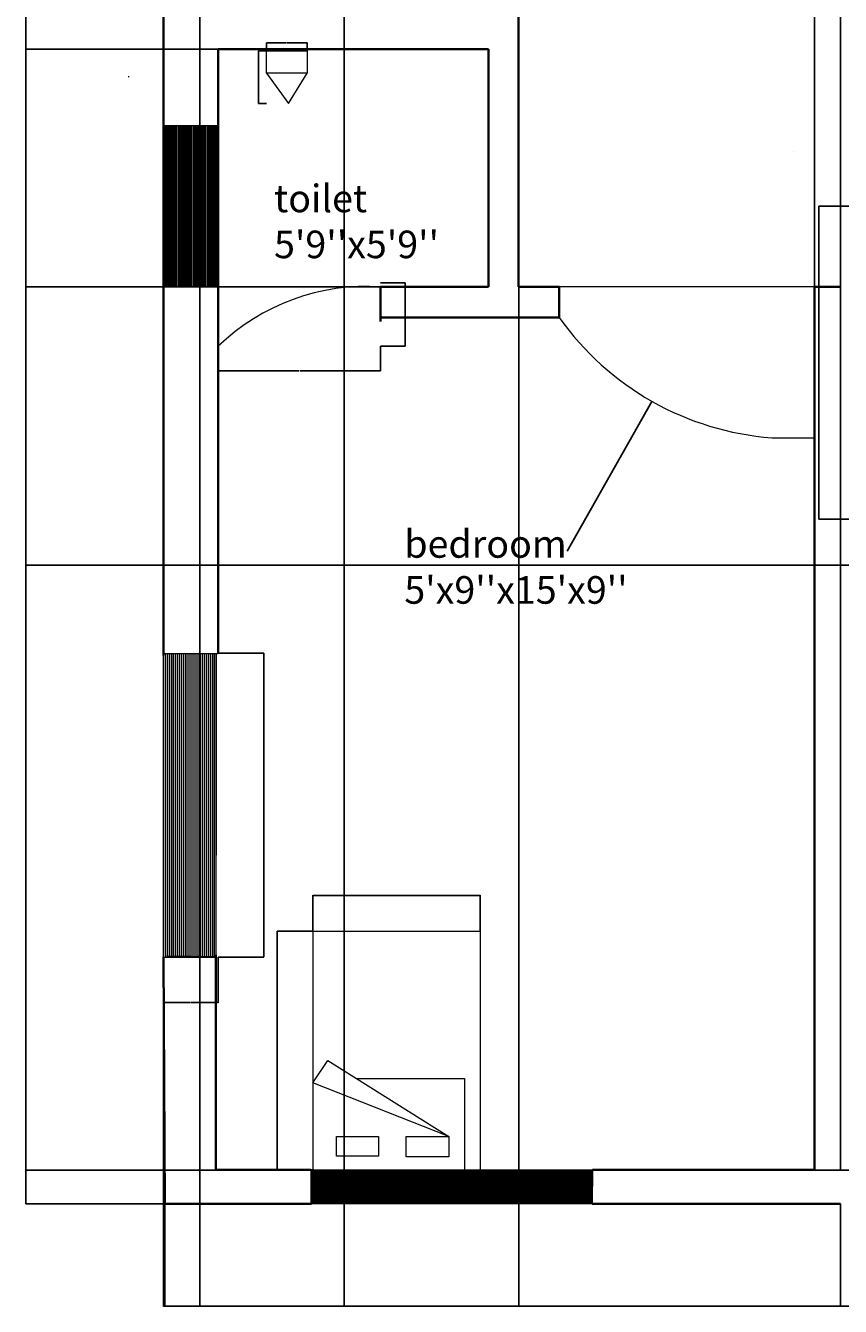
# Model space of a CAD drawing. Units: millimetres. Extents: x 1942 to 12281, y -2698 to 3078.
# Tile 1 of 6: x 1942 to 4011, y -2698 to 552. Entities that reach past the tile are written whole.
import ezdxf

# ---------------------------------------------------------------- set-up
doc = ezdxf.new("R2010")
doc.units = ezdxf.units.MM
for name, color, linetype, lineweight in [('A-ANNO-DIMS', 2, 'Continuous', 18), ('A-AREA-IDEN', 3, 'Continuous', 18), ('A-DETL-REF', 8, 'Continuous', 13), ('A-DOOR', 4, 'Continuous', 18), ('A-FLOR-FIXT', 9, 'Continuous', 18), ('A-FURN', 8, 'Continuous', 18), ('A-GLAZ', 4, 'Continuous', 18), ('A-GLAZ-PATT', 9, 'Continuous', 13), ('A-WALL', 7, 'Continuous', 35)]:
    doc.layers.add(name, color=color, linetype=linetype, lineweight=lineweight)
doc.styles.get("Standard").update_dxf_attribs({"font": 'arial.ttf'})
doc.dimstyles.get("Standard").update_dxf_attribs({"dimtxt": 0.18, "dimasz": 0.18, "dimexe": 0.18, "dimexo": 0.0625, "dimgap": 0.09, "dimtad": 0, "dimtih": 1, "dimtoh": 1, "dimdec": 4, "dimzin": 0, "dimdsep": 46, "dimtxsty": 'Standard', "dimcen": 0.09, "dimadec": 0, "dimazin": 0, "dimtfac": 1, "dimtdec": 4, "dimtofl": 0, "dimtmove": 0, "dimatfit": 3, "dimfxl": 1, "dimtolj": 1, "dimtzin": 0, "dimarcsym": 0})

# ---------------------------------------------------------------- blocks, each defined once
blk = doc.blocks.new('BED-PILLOWS')
for p, q in [((0, 605.9), (424.9, 605.9)), ((0, 605.9), (0, 0)), ((424.9, 605.9), (424.9, 0)), ((0, 221), (38.1, 277.4)), ((38.1, 277.4), (344.8, 84.6)), ((109.8, 232.4), (384.7, 232.4)), ((384.7, 232.4), (384.7, 0)), ((344.8, 84.6), (0, 221)), ((0, 0), (0, 0))]:
    blk.add_line(p, q)
for points in [[(59.7, 84.6), (166.4, 84.6), (166.4, 35.4), (59.7, 35.4)], [(236.8, 84.6), (344.8, 84.6), (344.8, 33.1), (236.8, 33.1)]]:
    blk.add_lwpolyline(points, close=True)
blk = doc.blocks.new('WC-TAPERED-LONG')
for p, q in [((0, 77), (55.9, 0)), ((55.9, 0), (103.2, 77))]:
    blk.add_line(p, q)
blk.add_lwpolyline([(0, 134), (103.2, 134), (103.2, 77), (0, 77)], close=True)
blk = doc.blocks.new('DOOR-BEDROOM')
for p, q in [((648.7, 382.9), (0, 382.9)), ((539.8, 0), (648.7, 0))]:
    blk.add_line(p, q)
blk.add_arc((594.3, 726.1), 728.1, 215.2982, 265.7132)
blk = doc.blocks.new('DOOR-WC-BEDROOM')
blk.add_arc((376.5, -390), 542.1, 86.1851, 133.9877)
blk = doc.blocks.new('WIN-BEDROOM-SIDE')
for p, q in [((138.7, 769.7), (0, 769.7)), ((0, 765.5), (0, 0.1)), ((132.6, 771), (132.6, 5.6)), ((0, 0.1), (132.6, 0.1)), ((8.8, 3.3), (132.6, 1.4)), ((95.6, 3.3), (78.2, 0))]:
    blk.add_line(p, q)
blk = doc.blocks.new('WIN-BEDROOM-END')
for p, q in [((0, 85.7), (0, 0)), ((0, 85.7), (430, 85.7)), ((714.9, 85.7), (714.3, 0)), ((714.3, 0), (1.8, 0))]:
    blk.add_line(p, q)
blk = doc.blocks.new('*D26')
at = {"layer": 'A-ANNO-DIMS', "color": 0, "lineweight": -2, "transparency": 16777216}
for p, q in [((2671.4, -1745.7), (2580.4, -1745.7)), ((2580.5, -1745.8), (2580.5, -2048.4)), ((2580.5, -2351.4), (2580.5, -2048.8)), ((2671.4, -2351.5), (2580.4, -2351.5))]:
    blk.add_line(p, q, dxfattribs=at)
at = {"layer": 'A-ANNO-DIMS', "color": 0, "transparency": 16777216}
for points in [[(2580.5, -1745.8), (2580.6, -1745.8), (2580.5, -1745.7)], [(2580.5, -2351.4), (2580.6, -2351.4), (2580.5, -2351.5)]]:
    blk.add_solid(points, dxfattribs=at)
at = {"layer": 'Defpoints', "color": 0, "transparency": 16777216}
for p in [(2580.5, -1745.7), (2671.4, -1745.7), (2671.4, -2351.5)]:
    blk.add_point(p, dxfattribs=at)
at = {"layer": 'A-ANNO-DIMS', "color": 0, "transparency": 16777216, "insert": (2580.5, -2048.6), "char_height": 0.18, "attachment_point": 5}
blk.add_mtext('\\A1;BED 606 TYP.', dxfattribs=at)
blk = doc.blocks.new('*D27')
at = {"layer": 'A-ANNO-DIMS', "color": 0, "lineweight": -2, "transparency": 16777216}
for p, q in [((2671.4, -1745.6), (2671.4, -1654.6)), ((2671.6, -1654.8), (2883.3, -1654.8)), ((3096.2, -1654.8), (2884.5, -1654.8)), ((3096.3, -1745.6), (3096.3, -1654.6))]:
    blk.add_line(p, q, dxfattribs=at)
at = {"layer": 'A-ANNO-DIMS', "color": 0, "transparency": 16777216}
for points in [[(2671.6, -1654.8), (2671.6, -1654.8), (2671.4, -1654.8)], [(3096.2, -1654.8), (3096.2, -1654.8), (3096.3, -1654.8)]]:
    blk.add_solid(points, dxfattribs=at)
at = {"layer": 'Defpoints', "color": 0, "transparency": 16777216}
for p in [(3096.3, -1654.8), (2671.4, -1745.7), (3096.3, -1745.7)]:
    blk.add_point(p, dxfattribs=at)
at = {"layer": 'A-ANNO-DIMS', "color": 0, "transparency": 16777216, "insert": (2883.9, -1654.8), "char_height": 0.18, "attachment_point": 5}
blk.add_mtext('\\A1;425 TYP.', dxfattribs=at)
blk = doc.blocks.new('*D29')
at = {"layer": 'A-ANNO-DIMS', "color": 0, "lineweight": -2, "transparency": 16777216}
for p, q in [((4101.3, 94.1), (3956.1, 94.1)), ((3956.3, 94), (3956.3, -302.8)), ((3956.3, -700), (3956.3, -303.2)), ((4101.3, -700.2), (3956.1, -700.2))]:
    blk.add_line(p, q, dxfattribs=at)
at = {"layer": 'A-ANNO-DIMS', "color": 0, "transparency": 16777216}
for points in [[(3956.3, 94), (3956.3, 94), (3956.3, 94.1)], [(3956.3, -700), (3956.3, -700), (3956.3, -700.2)]]:
    blk.add_solid(points, dxfattribs=at)
at = {"layer": 'Defpoints', "color": 0, "transparency": 16777216}
for p in [(3956.3, 94.1), (4101.4, 94.1), (4101.4, -700.2)]:
    blk.add_point(p, dxfattribs=at)
at = {"layer": 'A-ANNO-DIMS', "color": 0, "transparency": 16777216, "insert": (3956.3, -303), "char_height": 0.18, "attachment_point": 5}
blk.add_mtext('\\A1;794 TYP.', dxfattribs=at)
blk = doc.blocks.new('*D36')
at = {"layer": 'A-ANNO-DIMS', "color": 0, "lineweight": -2, "transparency": 16777216}
for p, q in [((2553.4, 488.5), (2533.2, 488.5)), ((2533.3, 488.3), (2533.3, 421.7)), ((2533.3, 354.7), (2533.3, 421.3)), ((2553.4, 354.5), (2533.2, 354.5))]:
    blk.add_line(p, q, dxfattribs=at)
at = {"layer": 'A-ANNO-DIMS', "color": 0, "transparency": 16777216}
for points in [[(2533.3, 488.3), (2533.4, 488.3), (2533.3, 488.5)], [(2533.3, 354.7), (2533.4, 354.7), (2533.3, 354.5)]]:
    blk.add_solid(points, dxfattribs=at)
at = {"layer": 'Defpoints', "color": 0, "transparency": 16777216}
for p in [(2533.3, 488.5), (2553.4, 488.5), (2553.4, 354.5)]:
    blk.add_point(p, dxfattribs=at)
at = {"layer": 'A-ANNO-DIMS', "color": 0, "transparency": 16777216, "insert": (2533.3, 421.5), "char_height": 0.18, "attachment_point": 5}
blk.add_mtext('\\A1;WC 134 TYP.', dxfattribs=at)
blk = doc.blocks.new('*D37')
at = {"layer": 'A-ANNO-DIMS', "color": 0, "lineweight": -2, "transparency": 16777216}
for p, q in [((2553.4, 488.5), (2553.4, 508.7)), ((2553.6, 508.6), (2604.4, 508.6)), ((2656.4, 508.6), (2605.6, 508.6)), ((2656.6, 488.5), (2656.6, 508.7))]:
    blk.add_line(p, q, dxfattribs=at)
at = {"layer": 'A-ANNO-DIMS', "color": 0, "transparency": 16777216}
for points in [[(2553.6, 508.6), (2553.6, 508.5), (2553.4, 508.6)], [(2656.4, 508.6), (2656.4, 508.5), (2656.6, 508.6)]]:
    blk.add_solid(points, dxfattribs=at)
at = {"layer": 'Defpoints', "color": 0, "transparency": 16777216}
for p in [(2553.4, 488.5), (2656.6, 508.6), (2656.6, 488.5)]:
    blk.add_point(p, dxfattribs=at)
at = {"layer": 'A-ANNO-DIMS', "color": 0, "transparency": 16777216, "insert": (2605, 508.6), "char_height": 0.18, "attachment_point": 5}
blk.add_mtext('\\A1;103 TYP.', dxfattribs=at)
blk = doc.blocks.new('*D44')
at = {"layer": 'A-ANNO-DIMS', "color": 0, "lineweight": -2, "transparency": 16777216}
for p, q in [((2430.7, -261.5), (2430.7, -323.5)), ((2843.3, -261.5), (2843.3, -323.5)), ((2430.9, -323.3), (2635.7, -323.3)), ((2843.1, -323.3), (2638.3, -323.3))]:
    blk.add_line(p, q, dxfattribs=at)
at = {"layer": 'A-ANNO-DIMS', "color": 0, "transparency": 16777216}
for points in [[(2430.9, -323.3), (2430.9, -323.4), (2430.7, -323.3)], [(2843.1, -323.3), (2843.1, -323.4), (2843.3, -323.3)]]:
    blk.add_solid(points, dxfattribs=at)
at = {"layer": 'Defpoints', "color": 0, "transparency": 16777216}
for p in [(2430.7, -261.5), (2843.3, -261.5), (2843.3, -323.3)]:
    blk.add_point(p, dxfattribs=at)
at = {"layer": 'A-ANNO-DIMS', "color": 0, "transparency": 16777216, "insert": (2637, -323.3), "char_height": 0.18, "attachment_point": 5}
blk.add_mtext('\\A1;WC DOOR 413 TYP.', dxfattribs=at)
blk = doc.blocks.new('*D45')
at = {"layer": 'A-ANNO-DIMS', "color": 0, "lineweight": -2, "transparency": 16777216}
for p, q in [((2843.3, -100.4), (2905.3, -100.4)), ((2905.2, -100.6), (2905.2, -180.8)), ((2905.2, -261.3), (2905.2, -181.1)), ((2843.3, -261.5), (2905.3, -261.5))]:
    blk.add_line(p, q, dxfattribs=at)
at = {"layer": 'A-ANNO-DIMS', "color": 0, "transparency": 16777216}
for points in [[(2905.1, -100.6), (2905.2, -100.6), (2905.2, -100.4)], [(2905.1, -261.3), (2905.2, -261.3), (2905.2, -261.5)]]:
    blk.add_solid(points, dxfattribs=at)
at = {"layer": 'Defpoints', "color": 0, "transparency": 16777216}
for p in [(2843.3, -100.4), (2905.2, -100.4), (2843.3, -261.5)]:
    blk.add_point(p, dxfattribs=at)
at = {"layer": 'A-ANNO-DIMS', "color": 0, "transparency": 16777216, "insert": (2905.2, -180.9), "char_height": 0.18, "attachment_point": 5}
blk.add_mtext('\\A1;161 TYP.', dxfattribs=at)
blk = doc.blocks.new('*D64')
at = {"layer": 'A-ANNO-DIMS', "color": 0, "lineweight": -2, "transparency": 16777216}
for p, q in [((2430.8, -1040.2), (2546.6, -1040.2)), ((2546.4, -1040.4), (2546.4, -1425.5)), ((2546.4, -1811), (2546.4, -1425.9)), ((2430.8, -1811.2), (2546.6, -1811.2))]:
    blk.add_line(p, q, dxfattribs=at)
at = {"layer": 'A-ANNO-DIMS', "color": 0, "transparency": 16777216}
for points in [[(2546.3, -1040.4), (2546.4, -1040.4), (2546.4, -1040.2)], [(2546.3, -1811), (2546.4, -1811), (2546.4, -1811.2)]]:
    blk.add_solid(points, dxfattribs=at)
at = {"layer": 'Defpoints', "color": 0, "transparency": 16777216}
for p in [(2430.7, -1040.2), (2546.4, -1040.2), (2430.7, -1811.2)]:
    blk.add_point(p, dxfattribs=at)
at = {"layer": 'A-ANNO-DIMS', "color": 0, "transparency": 16777216, "insert": (2546.4, -1425.7), "char_height": 0.18, "attachment_point": 5}
blk.add_mtext('\\A1;W3 771 TYP.', dxfattribs=at)
blk = doc.blocks.new('*D65')
at = {"layer": 'A-ANNO-DIMS', "color": 0, "lineweight": -2, "transparency": 16777216}
for p, q in [((2292.1, -1811.3), (2292.1, -1927)), ((2430.7, -1811.3), (2430.7, -1927)), ((2292.2, -1926.8), (2360.8, -1926.8)), ((2430.5, -1926.8), (2362, -1926.8))]:
    blk.add_line(p, q, dxfattribs=at)
at = {"layer": 'A-ANNO-DIMS', "color": 0, "transparency": 16777216}
for points in [[(2292.2, -1926.8), (2292.2, -1926.9), (2292.1, -1926.8)], [(2430.5, -1926.8), (2430.5, -1926.9), (2430.7, -1926.8)]]:
    blk.add_solid(points, dxfattribs=at)
at = {"layer": 'Defpoints', "color": 0, "transparency": 16777216}
for p in [(2292.1, -1811.2), (2430.7, -1811.2), (2430.7, -1926.8)]:
    blk.add_point(p, dxfattribs=at)
at = {"layer": 'A-ANNO-DIMS', "color": 0, "transparency": 16777216, "insert": (2361.4, -1926.8), "char_height": 0.18, "attachment_point": 5}
blk.add_mtext('\\A1;139 TYP.', dxfattribs=at)
blk = doc.blocks.new('*D72')
at = {"layer": 'A-ANNO-DIMS', "color": 0, "lineweight": -2, "transparency": 16777216}
for p, q in [((2295.7, -2437.3), (2295.7, -2697.7)), ((4010.7, -2437.3), (4010.7, -2697.7)), ((2295.8, -2697.5), (3152.8, -2697.5)), ((4010.5, -2697.5), (3153.5, -2697.5))]:
    blk.add_line(p, q, dxfattribs=at)
at = {"layer": 'A-ANNO-DIMS', "color": 0, "transparency": 16777216}
for points in [[(2295.8, -2697.5), (2295.8, -2697.5), (2295.7, -2697.5)], [(4010.5, -2697.5), (4010.5, -2697.5), (4010.7, -2697.5)]]:
    blk.add_solid(points, dxfattribs=at)
at = {"layer": 'Defpoints', "color": 0, "transparency": 16777216}
for p in [(2295.7, -2437.2), (4010.7, -2437.2), (4010.7, -2697.5)]:
    blk.add_point(p, dxfattribs=at)
at = {"layer": 'A-ANNO-DIMS', "color": 0, "transparency": 16777216, "insert": (3153.2, -2697.5), "char_height": 0.18, "attachment_point": 5}
blk.add_mtext('\\A1;1715', dxfattribs=at)
blk = doc.blocks.new('*D73')
at = {"layer": 'A-ANNO-DIMS', "color": 0, "lineweight": -2, "transparency": 16777216}
for p, q in [((4010.7, -2437.3), (4010.7, -2697.7)), ((6894.1, -2437.3), (6894.1, -2697.7)), ((4010.9, -2697.5), (5451.9, -2697.5)), ((6893.9, -2697.5), (5452.9, -2697.5))]:
    blk.add_line(p, q, dxfattribs=at)
at = {"layer": 'A-ANNO-DIMS', "color": 0, "transparency": 16777216}
for points in [[(4010.9, -2697.5), (4010.9, -2697.5), (4010.7, -2697.5)], [(6893.9, -2697.5), (6893.9, -2697.5), (6894.1, -2697.5)]]:
    blk.add_solid(points, dxfattribs=at)
at = {"layer": 'Defpoints', "color": 0, "transparency": 16777216}
for p in [(4010.7, -2437.2), (6894.1, -2437.2), (6894.1, -2697.5)]:
    blk.add_point(p, dxfattribs=at)
at = {"layer": 'A-ANNO-DIMS', "color": 0, "transparency": 16777216, "insert": (5452.4, -2697.5), "char_height": 0.18, "attachment_point": 5}
blk.add_mtext('\\A1;2883.4', dxfattribs=at)
blk = doc.blocks.new('*D77')
at = {"layer": 'A-ANNO-DIMS', "color": 0, "lineweight": -2, "transparency": 16777216}
for p, q in [((2292, 1112.1), (1942, 1112.1)), ((1942.2, 1111.9), (1942.2, 802.3)), ((1942.2, 492.4), (1942.2, 801.9)), ((3116.8, 492.2), (1942, 492.2))]:
    blk.add_line(p, q, dxfattribs=at)
at = {"layer": 'A-ANNO-DIMS', "color": 0, "transparency": 16777216}
for points in [[(1942.2, 1111.9), (1942.2, 1111.9), (1942.2, 1112.1)], [(1942.2, 492.4), (1942.2, 492.4), (1942.2, 492.2)]]:
    blk.add_solid(points, dxfattribs=at)
at = {"layer": 'Defpoints', "color": 0, "transparency": 16777216}
for p in [(1942.2, 1112.1), (2292.1, 1112.1), (3116.8, 492.2)]:
    blk.add_point(p, dxfattribs=at)
at = {"layer": 'A-ANNO-DIMS', "color": 0, "transparency": 16777216, "insert": (1942.2, 802.1), "char_height": 0.18, "attachment_point": 5}
blk.add_mtext('\\A1;619.9', dxfattribs=at)
blk = doc.blocks.new('*D78')
at = {"layer": 'A-ANNO-DIMS', "color": 0, "lineweight": -2, "transparency": 16777216}
for p, q in [((3116.8, 492.2), (1942, 492.2)), ((1942.2, 492), (1942.2, 191)), ((1942.2, -110.4), (1942.2, 190.6)), ((3116.8, -110.6), (1942, -110.6))]:
    blk.add_line(p, q, dxfattribs=at)
at = {"layer": 'A-ANNO-DIMS', "color": 0, "transparency": 16777216}
for points in [[(1942.2, 492), (1942.2, 492), (1942.2, 492.2)], [(1942.2, -110.4), (1942.2, -110.4), (1942.2, -110.6)]]:
    blk.add_solid(points, dxfattribs=at)
at = {"layer": 'Defpoints', "color": 0, "transparency": 16777216}
for p in [(1942.2, 492.2), (3116.8, 492.2), (3116.8, -110.6)]:
    blk.add_point(p, dxfattribs=at)
at = {"layer": 'A-ANNO-DIMS', "color": 0, "transparency": 16777216, "insert": (1942.2, 190.8), "char_height": 0.18, "attachment_point": 5}
blk.add_mtext('\\A1;602.8', dxfattribs=at)
blk = doc.blocks.new('*D79')
at = {"layer": 'A-ANNO-DIMS', "color": 0, "lineweight": -2, "transparency": 16777216}
for p, q in [((3116.8, -110.6), (1942, -110.6)), ((1942.2, -110.8), (1942.2, -1273.7)), ((1942.2, -2437.1), (1942.2, -1274.1)), ((2295.6, -2437.2), (1942, -2437.2))]:
    blk.add_line(p, q, dxfattribs=at)
at = {"layer": 'A-ANNO-DIMS', "color": 0, "transparency": 16777216}
for points in [[(1942.2, -110.8), (1942.2, -110.8), (1942.2, -110.6)], [(1942.2, -2437.1), (1942.2, -2437.1), (1942.2, -2437.2)]]:
    blk.add_solid(points, dxfattribs=at)
at = {"layer": 'Defpoints', "color": 0, "transparency": 16777216}
for p in [(1942.2, -110.6), (3116.8, -110.6), (2295.7, -2437.2)]:
    blk.add_point(p, dxfattribs=at)
at = {"layer": 'A-ANNO-DIMS', "color": 0, "transparency": 16777216, "insert": (1942.2, -1273.9), "char_height": 0.18, "attachment_point": 5}
blk.add_mtext('\\A1;2326.6', dxfattribs=at)
blk = doc.blocks.new('*D80')
at = {"layer": 'A-ANNO-DIMS', "color": 0, "lineweight": -2, "transparency": 16777216}
for p, q in [((2292.1, 1112), (2292.1, -2697.7)), ((3193.8, 769.3), (3193.8, -2697.7)), ((2292.2, -2697.5), (2742.5, -2697.5)), ((3193.6, -2697.5), (2743.3, -2697.5))]:
    blk.add_line(p, q, dxfattribs=at)
at = {"layer": 'A-ANNO-DIMS', "color": 0, "transparency": 16777216}
for points in [[(2292.2, -2697.5), (2292.2, -2697.5), (2292.1, -2697.5)], [(3193.6, -2697.5), (3193.6, -2697.5), (3193.8, -2697.5)]]:
    blk.add_solid(points, dxfattribs=at)
at = {"layer": 'Defpoints', "color": 0, "transparency": 16777216}
for p in [(2292.1, 1112.1), (3193.8, 769.4), (3193.8, -2697.5)]:
    blk.add_point(p, dxfattribs=at)
at = {"layer": 'A-ANNO-DIMS', "color": 0, "transparency": 16777216, "insert": (2742.9, -2697.5), "char_height": 0.18, "attachment_point": 5}
blk.add_mtext('\\A1;901.7', dxfattribs=at)
blk = doc.blocks.new('*D81')
at = {"layer": 'A-ANNO-DIMS', "color": 0, "lineweight": -2, "transparency": 16777216}
for p, q in [((6681.4, -817), (1942, -817)), ((1942.2, -817.2), (1942.2, -1584.1)), ((1942.2, -2351.4), (1942.2, -1584.5)), ((6681.4, -2351.6), (1942, -2351.6))]:
    blk.add_line(p, q, dxfattribs=at)
at = {"layer": 'A-ANNO-DIMS', "color": 0, "transparency": 16777216}
for points in [[(1942.2, -817.2), (1942.2, -817.2), (1942.2, -817)], [(1942.2, -2351.4), (1942.2, -2351.4), (1942.2, -2351.6)]]:
    blk.add_solid(points, dxfattribs=at)
at = {"layer": 'Defpoints', "color": 0, "transparency": 16777216}
for p in [(1942.2, -817), (6681.5, -817), (6681.5, -2351.6)]:
    blk.add_point(p, dxfattribs=at)
at = {"layer": 'A-ANNO-DIMS', "color": 0, "transparency": 16777216, "insert": (1942.2, -1584.3), "char_height": 0.18, "attachment_point": 5}
blk.add_mtext('\\A1;1534.5', dxfattribs=at)
blk = doc.blocks.new('*D85')
at = {"layer": 'A-ANNO-DIMS', "color": 0, "lineweight": -2, "transparency": 16777216}
for p, q in [((2384.1, 1439.1), (2384.1, -2697.7)), ((2750.5, 1439.1), (2750.5, -2697.7)), ((2384.3, -2697.5), (2566.9, -2697.5)), ((2750.3, -2697.5), (2567.7, -2697.5))]:
    blk.add_line(p, q, dxfattribs=at)
at = {"layer": 'A-ANNO-DIMS', "color": 0, "transparency": 16777216}
for points in [[(2384.3, -2697.5), (2384.3, -2697.5), (2384.1, -2697.5)], [(2750.3, -2697.5), (2750.3, -2697.5), (2750.5, -2697.5)]]:
    blk.add_solid(points, dxfattribs=at)
at = {"layer": 'Defpoints', "color": 0, "transparency": 16777216}
for p in [(2384.1, 1439.2), (2750.5, 1439.2), (2750.5, -2697.5)]:
    blk.add_point(p, dxfattribs=at)
at = {"layer": 'A-ANNO-DIMS', "color": 0, "transparency": 16777216, "insert": (2567.3, -2697.5), "char_height": 0.18, "attachment_point": 5}
blk.add_mtext('\\A1;366.4', dxfattribs=at)
blk = doc.blocks.new('*D89')
at = {"layer": 'A-ANNO-DIMS', "color": 0, "lineweight": -2, "transparency": 16777216}
for p, q in [((3945.3, -2351.5), (3945.3, 3026.3)), ((3945.5, 3026.1), (3977.7, 3026.1)), ((4010.5, 3026.1), (3978.3, 3026.1)), ((4010.7, -2351.5), (4010.7, 3026.3))]:
    blk.add_line(p, q, dxfattribs=at)
at = {"layer": 'A-ANNO-DIMS', "color": 0, "transparency": 16777216}
for points in [[(3945.5, 3026.2), (3945.5, 3026.1), (3945.3, 3026.1)], [(4010.5, 3026.2), (4010.5, 3026.1), (4010.7, 3026.1)]]:
    blk.add_solid(points, dxfattribs=at)
at = {"layer": 'Defpoints', "color": 0, "transparency": 16777216}
for p in [(4010.7, 3026.1), (3945.3, -2351.6), (4010.7, -2351.6)]:
    blk.add_point(p, dxfattribs=at)
at = {"layer": 'A-ANNO-DIMS', "color": 0, "transparency": 16777216, "insert": (3978, 3026.1), "char_height": 0.18, "attachment_point": 5}
blk.add_mtext('\\A1;65.4', dxfattribs=at)
blk = doc.blocks.new('*D115')
at = {"layer": 'A-ANNO-DIMS', "color": 0, "lineweight": -2, "transparency": 16777216}
for p, q in [((3890.8, 232.6), (3891, 232.6)), ((3890.9, 232.5), (3890.9, 232.7)), ((3317.3, -781.4), (3532.3, -401.3)), ((3317.1, -781.4), (3317.3, -781.4))]:
    blk.add_line(p, q, dxfattribs=at)
at = {"layer": 'A-ANNO-DIMS', "color": 0, "transparency": 16777216}
blk.add_solid([(3532.3, -401.3), (3532.3, -401.3), (3532.4, -401.1)], dxfattribs=at)
at = {"layer": 'Defpoints', "color": 0, "transparency": 16777216}
for p in [(3890.9, 232.6), (3532.4, -401.1)]:
    blk.add_point(p, dxfattribs=at)
at = {"layer": 'A-ANNO-DIMS', "color": 0, "transparency": 16777216, "insert": (3316.5, -781.4), "char_height": 0.18, "attachment_point": 5}
blk.add_mtext('\\A1;2X R728.1', dxfattribs=at)

msp = doc.modelspace()

# ---------------------------------------------------------------- hatches: boundary and pattern name
at = {"layer": 'A-GLAZ-PATT'}
h = msp.add_hatch(dxfattribs=at)
h.set_pattern_fill('ANSI31', color=256, scale=1.091886, angle=45, style=0)
h.paths.add_polyline_path([(2292.051, -110.599), (2430.72, -110.599), (2430.72, 298.853), (2292.051, 298.853)])
h = msp.add_hatch(dxfattribs=at)
h.set_pattern_fill('ANSI31', color=256, scale=1.559837, angle=45, style=0)
h.paths.add_polyline_path([(2292.051, -1811.074), (2424.694, -1811.074), (2430.72, -1041.509), (2292.051, -1041.509)])
h = msp.add_hatch(dxfattribs=at)
h.set_pattern_fill('ANSI31', color=256, scale=0.870611, angle=135, style=0)
h.paths.add_polyline_path([(2666.365, -2437.233), (3380.631, -2437.233), (3381.261, -2351.545), (2666.365, -2351.543)])

# ---------------------------------------------------------------- linework, layer by layer
at = {"layer": 'A-DETL-REF'}
for p, q in [((2204.95, 422.273), (2202.45, 422.273)), ((2513.372, -1811.074), (2513.372, -1811.074))]:
    msp.add_line(p, q, dxfattribs=at)
at = {"layer": 'A-GLAZ'}
for p, q in [((2292.051, 298.853), (2430.72, 298.853)), ((2292.051, -110.599), (2430.72, -110.599))]:
    msp.add_line(p, q, dxfattribs=at)
at = {"layer": 'A-WALL'}
for p, q in [((3193.761, 769.368), (3193.761, 44.982)), ((2292.051, 741.277), (2292.051, 298.853)), ((2430.72, 298.853), (2430.72, 492.199)), ((2430.72, 492.199), (2652.11, 492.199)), ((2652.11, 492.199), (2967.937, 492.199)), ((2967.937, 492.199), (3116.85, 492.199)), ((3116.85, 492.199), (3116.85, 38.441)), ((2292.051, 298.853), (2292.051, 298.853)), ((2292.051, 298.853), (2292.051, -1045.713)), ((2430.72, 298.853), (2430.72, -1041.509)), ((3116.85, 38.441), (3116.85, -110.599)), ((3193.761, 44.982), (3193.761, -110.599)), ((2843.269, -110.599), (3116.85, -110.599)), ((2843.269, -110.599), (2843.269, -198.495)), ((3193.761, -110.599), (3296.624, -110.599)), ((3296.624, -110.599), (3296.624, -110.599)), ((3296.624, -110.599), (3296.624, -188.119)), ((3945.31, -1017.162), (3945.31, -110.599)), ((3945.31, -110.599), (4010.712, -110.599)), ((3296.624, -188.119), (2843.269, -188.119)), ((3945.31, -2351.554), (3945.31, -1017.162)), ((2292.051, -1811.074), (2295.658, -2437.233)), ((2424.694, -1805.552), (2424.694, -2351.543)), ((2424.694, -2351.543), (2666.365, -2351.543)), ((3381.261, -2351.545), (3945.31, -2351.554)), ((2295.658, -2437.233), (2668.115, -2437.233)), ((3380.631, -2437.233), (4010.712, -2437.233))]:
    msp.add_line(p, q, dxfattribs=at)

# ---------------------------------------------------------------- block references
at = {"layer": 'A-DOOR'}
for name, p in [('DOOR-WC-BEDROOM', (2430.72, -261.46)), ('DOOR-BEDROOM', (3296.624, -493.47))]:
    msp.add_blockref(name, p, dxfattribs=at)
at = {"layer": 'A-FLOR-FIXT'}
msp.add_blockref('WC-TAPERED-LONG', (2553.44, 354.516), dxfattribs=at)
at = {"layer": 'A-FURN'}
msp.add_blockref('BED-PILLOWS', (2671.416, -2351.543), dxfattribs=at)
at = {"layer": 'A-GLAZ'}
for name, p in [('WIN-BEDROOM-SIDE', (2292.051, -1811.196)), ('WIN-BEDROOM-END', (2666.365, -2437.233))]:
    msp.add_blockref(name, p, dxfattribs=at)

# ---------------------------------------------------------------- texts
at = {"layer": 'A-AREA-IDEN', "insert": (2572.702, 148.795), "char_height": 70, "attachment_point": 1}
msp.add_mtext("toilet\\P5'9''x5'9''", dxfattribs=at)
at = {"layer": 'A-AREA-IDEN', "insert": (2903.475, -727.987), "char_height": 70, "attachment_point": 1}
msp.add_mtext_dynamic_manual_height_columns("bedroom\\P5'x9''x15'x9''", width=79.60101, gutter_width=12.5, heights=[0], dxfattribs=at)

# ---------------------------------------------------------------- dimensions: what is measured, and where the dimension line sits
at = {"layer": 'A-ANNO-DIMS'}
for base, p1, p2, override, picture, middle in [((4010.712, 3026.123), (3945.31, -2351.554), (4010.712, -2351.554), {"dimdec": 1, "dimlfac": 1, "dimrnd": 0, "dimzin": 0, "dimdsep": 46, "dimlunit": 2}, '*D89', (3978.011, 3026.123)), ((2750.504, -2697.483), (2384.129, 1439.211), (2750.504, 1439.211), {"dimdec": 1, "dimlfac": 1, "dimrnd": 0, "dimzin": 0, "dimdsep": 46, "dimlunit": 2}, '*D85', (2567.317, -2697.483)), ((3193.761, -2697.483), (2292.051, 1112.062), (3193.761, 769.368), {"dimdec": 1, "dimlfac": 1, "dimrnd": 0, "dimzin": 0, "dimdsep": 46, "dimlunit": 2}, '*D80', (2742.906, -2697.483)), ((4010.712, -2697.483), (2295.658, -2437.233), (4010.712, -2437.233), {"dimdec": 0, "dimlfac": 1, "dimrnd": 0, "dimzin": 0, "dimdsep": 46, "dimlunit": 2}, '*D72', (3153.185, -2697.483)), ((6894.096, -2697.483), (4010.712, -2437.233), (6894.096, -2437.233), {"dimdec": 1, "dimlfac": 1, "dimrnd": 0, "dimzin": 0, "dimdsep": 46, "dimlunit": 2}, '*D73', (5452.404, -2697.483))]:
    dim = msp.add_linear_dim(base=base, p1=p1, p2=p2, dimstyle='Standard', override=override, dxfattribs=at)
    dim.commit()
    dim.dimension.update_dxf_attribs({"geometry": picture, "text_midpoint": middle})
for base, p1, p2, picture, middle in [((1942.2, 1112.062), (3116.85, 492.199), (2292.051, 1112.062), '*D77', (1942.2, 802.131)), ((1942.2, 492.199), (3116.85, -110.599), (3116.85, 492.199), '*D78', (1942.2, 190.8)), ((1942.2, -110.599), (2295.658, -2437.233), (3116.85, -110.599), '*D79', (1942.2, -1273.916)), ((1942.2, -817.04), (6681.459, -2351.554), (6681.459, -817.04), '*D81', (1942.2, -1584.297))]:
    dim = msp.add_linear_dim(base=base, p1=p1, p2=p2, angle=90, dimstyle='Standard', override={"dimdec": 1, "dimlfac": 1, "dimrnd": 0, "dimzin": 0, "dimdsep": 46, "dimlunit": 2}, dxfattribs=at)
    dim.commit()
    dim.dimension.update_dxf_attribs({"geometry": picture, "text_midpoint": middle})
for base, p1, p2, text, picture, middle in [((2533.347, 488.467), (2553.44, 354.516), (2553.44, 488.467), 'WC <> TYP.', '*D36', (2533.347, 421.492)), ((3956.289, 94.15), (4101.403, -700.178), (4101.403, 94.15), '<> TYP.', '*D29', (3956.289, -303.014)), ((2905.151, -100.421), (2843.269, -261.46), (2843.269, -100.421), '<> TYP.', '*D45', (2905.151, -180.94)), ((2546.371, -1040.19), (2430.72, -1811.196), (2430.72, -1040.19), 'W3 <> TYP.', '*D64', (2546.371, -1425.693)), ((2580.535, -1745.667), (2671.416, -2351.543), (2671.416, -1745.667), 'BED <> TYP.', '*D26', (2580.535, -2048.605))]:
    dim = msp.add_linear_dim(base=base, p1=p1, p2=p2, angle=90, text=text, dimstyle='Standard', override={"dimdec": 0, "dimlfac": 1, "dimrnd": 0, "dimzin": 0, "dimdsep": 46, "dimlunit": 2}, dxfattribs=at)
    dim.commit()
    dim.dimension.update_dxf_attribs({"geometry": picture, "text_midpoint": middle})
for base, p1, p2, text, picture, middle in [((2656.625, 508.56), (2553.44, 488.467), (2656.625, 488.467), '<> TYP.', '*D37', (2605.033, 508.56)), ((2843.269, -323.342), (2430.72, -261.46), (2843.269, -261.46), 'WC DOOR <> TYP.', '*D44', (2636.994, -323.342)), ((3096.338, -1654.786), (2671.416, -1745.667), (3096.338, -1745.667), '<> TYP.', '*D27', (2883.877, -1654.786)), ((2430.72, -1926.847), (2292.051, -1811.196), (2430.72, -1811.196), '<> TYP.', '*D65', (2361.385, -1926.847))]:
    dim = msp.add_linear_dim(base=base, p1=p1, p2=p2, text=text, dimstyle='Standard', override={"dimdec": 0, "dimlfac": 1, "dimrnd": 0, "dimzin": 0, "dimdsep": 46, "dimlunit": 2}, dxfattribs=at)
    dim.commit()
    dim.dimension.update_dxf_attribs({"geometry": picture, "text_midpoint": middle})
dim = msp.add_radius_dim(center=(3890.883, 232.613), mpoint=(3532.402, -401.146), text='2X <>', dimstyle='Standard', override={"dimdec": 1, "dimlfac": 1, "dimrnd": 0, "dimzin": 0, "dimdsep": 46, "dimlunit": 2}, dxfattribs=at)
dim.commit()
dim.dimension.update_dxf_attribs({"geometry": '*D115', "text_midpoint": (3316.476, -781.401), "dimtype": 164})

doc.saveas('drawing.dxf')
